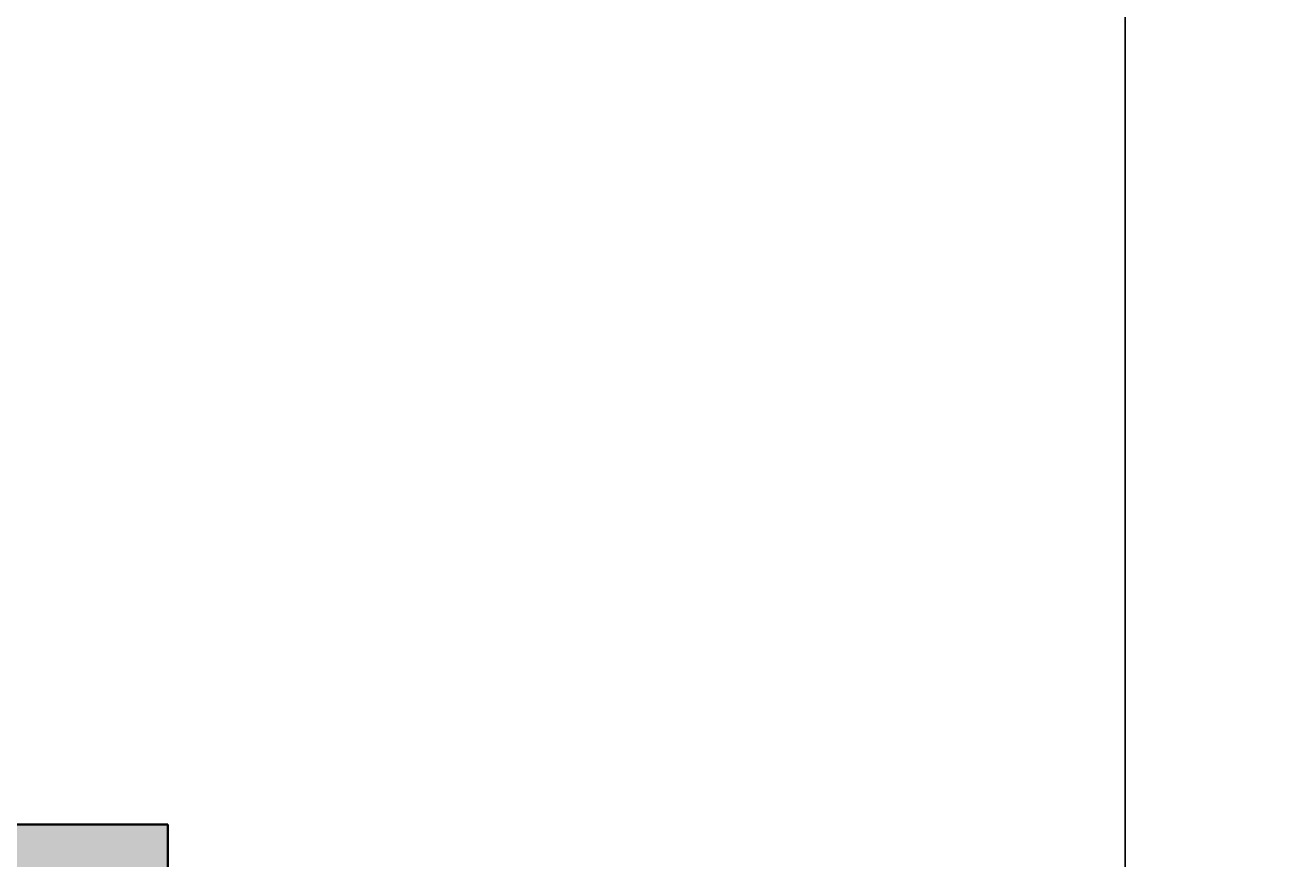
# Model space of a CAD drawing. Units: inches. Extents: x -301 to 715, y -607 to 364.
# Tile 10 of 141: x -19 to 18, y -536 to -512. Entities that reach past the tile are written whole.
import ezdxf

# ---------------------------------------------------------------- set-up
doc = ezdxf.new("R2010")
doc.units = ezdxf.units.IN
doc.header["$MEASUREMENT"] = 0
for name, color, linetype, lineweight in [('A-ANNO-DIMS', 2, 'Continuous', 18), ('A-SECT-PATT', 8, 'Continuous', 13), ('S-FNDN', 2, 'Continuous', 35)]:
    doc.layers.add(name, color=color, linetype=linetype, lineweight=lineweight)
doc.styles.get("Standard").update_dxf_attribs({"font": 'arial.ttf'})
doc.dimstyles.get("Standard").update_dxf_attribs({"dimtxt": 0.18, "dimasz": 0.18, "dimexe": 0.18, "dimexo": 0.0625, "dimgap": 0.09, "dimtad": 0, "dimtih": 1, "dimtoh": 1, "dimdec": 1, "dimzin": 0, "dimdsep": 46, "dimlunit": 4, "dimtxsty": 'Standard', "dimcen": 0.09, "dimclrd": 3, "dimclre": 4, "dimclrt": 6, "dimadec": 0, "dimazin": 0, "dimtfac": 1, "dimtdec": 1, "dimtofl": 0, "dimtmove": 0, "dimatfit": 3, "dimfxl": 1, "dimtfill": 2, "dimtfillclr": 51, "dimtolj": 1, "dimtzin": 0, "dimarcsym": 0})

# ---------------------------------------------------------------- blocks, each defined once
blk = doc.blocks.new('*D176')
at = {"layer": 'A-ANNO-DIMS', "color": 4, "lineweight": -2, "transparency": 16777216}
for p, q in [((148.28, -324.477), (215.605, -324.477)), ((-15.22, -540.477), (215.605, -540.477))]:
    blk.add_line(p, q, dxfattribs=at)
at = {"layer": 'A-ANNO-DIMS', "color": 3, "lineweight": -2, "transparency": 16777216}
for p, q in [((215.425, -324.657), (215.425, -432.296)), ((215.425, -540.297), (215.425, -432.659))]:
    blk.add_line(p, q, dxfattribs=at)
at = {"layer": 'A-ANNO-DIMS', "color": 3, "transparency": 16777216}
for points in [[(215.395, -324.657), (215.455, -324.657), (215.425, -324.477)], [(215.395, -540.297), (215.455, -540.297), (215.425, -540.477)]]:
    blk.add_solid(points, dxfattribs=at)
at = {"layer": 'Defpoints', "color": 0, "transparency": 16777216}
for p in [(148.218, -324.477), (-15.282, -540.477), (215.425, -540.477)]:
    blk.add_point(p, dxfattribs=at)
at = {"layer": 'A-ANNO-DIMS', "color": 6, "transparency": 16777216, "insert": (215.425, -432.477), "char_height": 0.18, "attachment_point": 5, "bg_fill": 1, "box_fill_scale": 1.25, "bg_fill_color": 51, "bg_fill_transparency": 0}
blk.add_mtext('\\A1;18\'-0"', dxfattribs=at)
blk = doc.blocks.new('*D180')
at = {"layer": 'A-ANNO-DIMS', "color": 4, "lineweight": -2, "transparency": 16777216}
for p, q in [((-35.282, -463.54), (-35.282, -573.809)), ((12.718, -463.54), (12.718, -573.809))]:
    blk.add_line(p, q, dxfattribs=at)
at = {"layer": 'A-ANNO-DIMS', "color": 3, "lineweight": -2, "transparency": 16777216}
for p, q in [((-35.102, -573.629), (-11.615, -573.629)), ((12.538, -573.629), (-10.949, -573.629))]:
    blk.add_line(p, q, dxfattribs=at)
at = {"layer": 'A-ANNO-DIMS', "color": 3, "transparency": 16777216}
for points in [[(-35.102, -573.599), (-35.102, -573.659), (-35.282, -573.629)], [(12.538, -573.599), (12.538, -573.659), (12.718, -573.629)]]:
    blk.add_solid(points, dxfattribs=at)
at = {"layer": 'Defpoints', "color": 0, "transparency": 16777216}
for p in [(-35.282, -463.477), (12.718, -463.477), (12.718, -573.629)]:
    blk.add_point(p, dxfattribs=at)
at = {"layer": 'A-ANNO-DIMS', "color": 6, "transparency": 16777216, "insert": (-11.282, -573.629), "char_height": 0.18, "attachment_point": 5, "bg_fill": 1, "box_fill_scale": 1.25, "bg_fill_color": 51, "bg_fill_transparency": 0}
blk.add_mtext('\\A1;4\'-0"', dxfattribs=at)
blk = doc.blocks.new('*D181')
at = {"layer": 'A-ANNO-DIMS', "color": 4, "lineweight": -2, "transparency": 16777216}
for p, q in [((48.468, -433.54), (48.468, -573.809)), ((12.718, -463.54), (12.718, -573.809))]:
    blk.add_line(p, q, dxfattribs=at)
at = {"layer": 'A-ANNO-DIMS', "color": 3, "lineweight": -2, "transparency": 16777216}
for p, q in [((12.898, -573.629), (30.264, -573.629)), ((48.288, -573.629), (30.922, -573.629))]:
    blk.add_line(p, q, dxfattribs=at)
at = {"layer": 'A-ANNO-DIMS', "color": 3, "transparency": 16777216}
for points in [[(12.898, -573.599), (12.898, -573.659), (12.718, -573.629)], [(48.288, -573.599), (48.288, -573.659), (48.468, -573.629)]]:
    blk.add_solid(points, dxfattribs=at)
at = {"layer": 'Defpoints', "color": 0, "transparency": 16777216}
for p in [(48.468, -433.477), (12.718, -463.477), (48.468, -573.629)]:
    blk.add_point(p, dxfattribs=at)
at = {"layer": 'A-ANNO-DIMS', "color": 6, "transparency": 16777216, "insert": (30.593, -573.629), "char_height": 0.18, "attachment_point": 5, "bg_fill": 1, "box_fill_scale": 1.25, "bg_fill_color": 51, "bg_fill_transparency": 0}
blk.add_mtext('\\A1;3\'-0"', dxfattribs=at)
blk = doc.blocks.new('*D191')
at = {"layer": 'A-ANNO-DIMS', "color": 4, "lineweight": -2, "transparency": 16777216}
for p, q in [((129.193, -481.477), (-266.112, -481.477)), ((114.193, -540.477), (-266.112, -540.477))]:
    blk.add_line(p, q, dxfattribs=at)
at = {"layer": 'A-ANNO-DIMS', "color": 3, "lineweight": -2, "transparency": 16777216}
for p, q in [((-265.932, -481.657), (-265.932, -510.797)), ((-265.932, -540.297), (-265.932, -511.158))]:
    blk.add_line(p, q, dxfattribs=at)
at = {"layer": 'A-ANNO-DIMS', "color": 3, "transparency": 16777216}
for points in [[(-265.962, -481.657), (-265.902, -481.657), (-265.932, -481.477)], [(-265.962, -540.297), (-265.902, -540.297), (-265.932, -540.477)]]:
    blk.add_solid(points, dxfattribs=at)
at = {"layer": 'Defpoints', "color": 0, "transparency": 16777216}
for p in [(129.255, -481.477), (-265.932, -540.477), (114.255, -540.477)]:
    blk.add_point(p, dxfattribs=at)
at = {"layer": 'A-ANNO-DIMS', "color": 6, "transparency": 16777216, "insert": (-265.932, -510.977), "char_height": 0.18, "attachment_point": 5, "bg_fill": 1, "box_fill_scale": 1.25, "bg_fill_color": 51, "bg_fill_transparency": 0}
blk.add_mtext('\\A1;4\'-11"', dxfattribs=at)

msp = doc.modelspace()

# ---------------------------------------------------------------- hatches: boundary and pattern name
at = {"layer": 'A-SECT-PATT'}
h = msp.add_hatch(dxfattribs=at)
h.set_pattern_fill('AR-CONC', color=256, scale=0.5)
h.set_pattern_definition([(50, (10.3213, 33.8764), (3.586301, -0.31376), [0.375, -4.125]), (355, (10.3213, 33.8764), (-0.693757, 3.76096), [0.3, -3.3]), (100.45144, (10.62, 33.8502), (2.892544, 3.4472), [0.3187, -3.50571]), (46.1842, (10.3213, 34.8764), (5.336207, -0.827596), [0.5625, -6.1875]), (96.6356, (10.766, 34.8074), (4.67331, 4.870593), [0.47805, -5.25857]), (351.1842, (10.321, 34.8764), (4.67331, 4.870593), [0.45, -4.95]), (21, (10.8213, 34.6264), (2.984535, -2.013094), [0.375, -4.125]), (326, (10.8213, 34.6264), (1.216577, 3.62575), [0.3, -3.3]), (71.45144, (11.07, 34.4586), (4.201112, 1.612656), [0.3187, -3.50571]), (37.5, (10.3213, 33.8764), (0.0607993, 1.6644693), [0, -3.26, 0, -3.35, 0, -3.3125]), (7.5, (10.3213, 33.8764), (1.3153477, 1.9720586), [0, -1.91, 0, -3.185, 0, -1.2625]), (327.5, (9.2063, 33.8764), (2.6691122, -0.1127744), [0, -1.25, 0, -3.9, 0, -5.175]), (317.5, (8.7063, 33.8764), (2.915931, 0.500525), [0, -1.625, 0, -2.59, 0, -3.675])])
h.paths.add_polyline_path([(-56.282, -535.477), (-61.282, -535.477), (-61.282, -540.477), (-15.282, -540.477), (-15.282, -535.477), (-20.282, -535.477)])
h.paths.add_polyline_path([(119.255, -535.477), (114.255, -535.477), (114.255, -540.477), (163.255, -540.477), (163.255, -535.477), (158.255, -535.477)])
h.paths.add_polyline_path([(-206.282, -471.477), (-209.282, -471.477), (-209.282, -481.477), (-206.282, -481.477), (-194.282, -481.477), (-194.282, -471.477)])
h.paths.add_polyline_path([(-41.282, -481.477), (-41.282, -471.477), (-185.282, -471.477), (-185.282, -481.477), (-180.282, -481.477)])
h.paths.add_polyline_path([(134.255, -481.477), (134.255, -471.477), (-35.282, -471.477), (-35.282, -481.477), (-30.282, -481.477)])
h.paths.add_polyline_path([(155.218, -481.477), (158.218, -481.477), (158.218, -471.477), (153.218, -471.477), (143.218, -471.477), (143.218, -481.477), (148.255, -481.477)])
h.paths.add_polyline_path([(-193.88, -356.477), (-193.904, -361.477), (143.218, -361.477), (143.218, -356.477)])

# ---------------------------------------------------------------- linework, layer by layer
at = {"layer": 'S-FNDN'}
for p, q in [((-20.282, -535.477), (-15.282, -535.477)), ((-15.282, -535.477), (-15.282, -540.477))]:
    msp.add_line(p, q, dxfattribs=at)

# ---------------------------------------------------------------- dimensions: what is measured, and where the dimension line sits
at = {"layer": 'A-ANNO-DIMS'}
for base, p1, p2, picture, middle in [((215.425, -540.477), (148.218, -324.477), (-15.282, -540.477), '*D176', (215.425, -432.477)), ((-265.932, -540.477), (129.255, -481.477), (114.255, -540.477), '*D191', (-265.932, -510.977))]:
    dim = msp.add_linear_dim(base=base, p1=p1, p2=p2, angle=90, dimstyle='Standard', override={"dimdec": 1, "dimlfac": 1, "dimrnd": 0, "dimzin": 1, "dimdsep": 46, "dimlunit": 4, "dimfrac": 2}, dxfattribs=at)
    dim.commit()
    dim.dimension.update_dxf_attribs({"geometry": picture, "text_midpoint": middle})
for base, p1, p2, picture, middle in [((48.467984, -573.628877), (12.717984, -463.47741), (48.467984, -433.47741), '*D181', (30.592984, -573.628877)), ((12.718, -573.629), (-35.282, -463.477), (12.718, -463.477), '*D180', (-11.282, -573.629))]:
    dim = msp.add_linear_dim(base=base, p1=p1, p2=p2, dimstyle='Standard', override={"dimdec": 1, "dimlfac": 1, "dimrnd": 0, "dimzin": 1, "dimdsep": 46, "dimlunit": 4, "dimfrac": 2}, dxfattribs=at)
    dim.commit()
    dim.dimension.update_dxf_attribs({"geometry": picture, "text_midpoint": middle})

doc.saveas('drawing.dxf')
